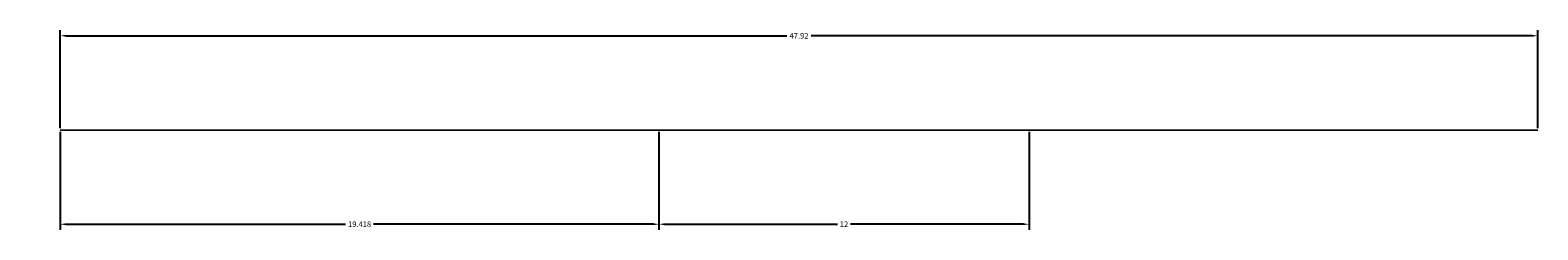
# Model space of a CAD drawing. Units: millimetres. Extents: x 4631 to 4863, y -3 to 1956.
# Tile 1 of 2: x 4814 to 4863, y -3 to 3. Entities that reach past the tile are written whole.
import ezdxf

# ---------------------------------------------------------------- set-up
doc = ezdxf.new("R2010")
doc.units = ezdxf.units.MM
doc.layers.add('M-CONS', color=8, linetype='Continuous', lineweight=13)
doc.layers.add('M-DIMS', color=2, linetype='Continuous', lineweight=18)
doc.styles.get("Standard").update_dxf_attribs({"font": 'arial.ttf'})
doc.dimstyles.get("Standard").update_dxf_attribs({"dimtxt": 0.18, "dimasz": 0.18, "dimexe": 0.18, "dimexo": 0.0625, "dimgap": 0.09, "dimtad": 0, "dimtih": 1, "dimtoh": 1, "dimdec": 4, "dimzin": 0, "dimdsep": 46, "dimtxsty": 'Standard', "dimcen": 0.09, "dimadec": 0, "dimazin": 0, "dimtfac": 1, "dimtdec": 4, "dimtofl": 0, "dimtmove": 0, "dimatfit": 3, "dimfxl": 1, "dimtolj": 1, "dimtzin": 0, "dimarcsym": 0})

# ---------------------------------------------------------------- blocks, each defined once
blk = doc.blocks.new('*D1')
at = {"layer": 'Defpoints', "color": 0, "transparency": 16777216}
for p in [(4863.262, 3.05), (4815.344, 0), (4863.262, 0)]:
    blk.add_point(p, dxfattribs=at)
at = {"layer": 'M-DIMS', "color": 0, "lineweight": -2, "transparency": 16777216}
for p, q in [((4815.344, 0.062), (4815.344, 3.23)), ((4815.524, 3.05), (4838.906, 3.05)), ((4863.082, 3.05), (4839.699, 3.05)), ((4863.262, 0.062), (4863.262, 3.23))]:
    blk.add_line(p, q, dxfattribs=at)
at = {"layer": 'M-DIMS', "color": 0, "transparency": 16777216}
for points in [[(4815.524, 3.08), (4815.524, 3.02), (4815.344, 3.05)], [(4863.082, 3.08), (4863.082, 3.02), (4863.262, 3.05)]]:
    blk.add_solid(points, dxfattribs=at)
at = {"layer": 'M-DIMS', "color": 0, "transparency": 16777216, "insert": (4839.303, 3.05), "char_height": 0.18, "attachment_point": 5}
blk.add_mtext('\\A1;47.92', dxfattribs=at)
blk = doc.blocks.new('*D2')
at = {"layer": 'Defpoints', "color": 0, "transparency": 16777216}
for p in [(4815.344, 0), (4834.762, 0), (4834.762, -3.05)]:
    blk.add_point(p, dxfattribs=at)
at = {"layer": 'M-DIMS', "color": 0, "lineweight": -2, "transparency": 16777216}
for p, q in [((4815.344, -0.062), (4815.344, -3.23)), ((4834.762, -0.062), (4834.762, -3.23)), ((4815.524, -3.05), (4824.597, -3.05)), ((4834.582, -3.05), (4825.508, -3.05))]:
    blk.add_line(p, q, dxfattribs=at)
at = {"layer": 'M-DIMS', "color": 0, "transparency": 16777216}
for points in [[(4815.524, -3.02), (4815.524, -3.08), (4815.344, -3.05)], [(4834.582, -3.02), (4834.582, -3.08), (4834.762, -3.05)]]:
    blk.add_solid(points, dxfattribs=at)
at = {"layer": 'M-DIMS', "color": 0, "transparency": 16777216, "insert": (4825.053, -3.05), "char_height": 0.18, "attachment_point": 5}
blk.add_mtext('\\A1;19.418', dxfattribs=at)
blk = doc.blocks.new('*D3')
at = {"layer": 'Defpoints', "color": 0, "transparency": 16777216}
for p in [(4834.762, 0), (4846.762, 0), (4846.762, -3.05)]:
    blk.add_point(p, dxfattribs=at)
at = {"layer": 'M-DIMS', "color": 0, "lineweight": -2, "transparency": 16777216}
for p, q in [((4834.762, -0.062), (4834.762, -3.23)), ((4846.762, -0.062), (4846.762, -3.23)), ((4834.942, -3.05), (4840.552, -3.05)), ((4846.582, -3.05), (4840.971, -3.05))]:
    blk.add_line(p, q, dxfattribs=at)
at = {"layer": 'M-DIMS', "color": 0, "transparency": 16777216}
for points in [[(4834.942, -3.02), (4834.942, -3.08), (4834.762, -3.05)], [(4846.582, -3.02), (4846.582, -3.08), (4846.762, -3.05)]]:
    blk.add_solid(points, dxfattribs=at)
at = {"layer": 'M-DIMS', "color": 0, "transparency": 16777216, "insert": (4840.762, -3.05), "char_height": 0.18, "attachment_point": 5}
blk.add_mtext('\\A1;12', dxfattribs=at)

msp = doc.modelspace()

# ---------------------------------------------------------------- linework, layer by layer
at = {"layer": 'M-CONS', "extrusion": (0, -1, 0)}
msp.add_lwpolyline([(4863.2618, -92.5722), (4818.2618, -92.5722, 0.145898), (4818.2618, -132.5722), (4863.2618, -132.5722)], format="xyb", close=True, dxfattribs=at)
msp.add_circle((4840.7618, -112.5722), 6, dxfattribs=at)

# ---------------------------------------------------------------- dimensions: what is measured, and where the dimension line sits
at = {"layer": 'M-DIMS'}
for base, p1, p2, override, picture, middle in [((4863.2618, 3.05), (4815.3438, 0), (4863.2618, 0), {"dimdec": 2, "dimlfac": 1, "dimrnd": 0, "dimzin": 0, "dimdsep": 46, "dimlunit": 2}, '*D1', (4839.3028, 3.05)), ((4834.7618, -3.05), (4815.3438, 0), (4834.7618, 0), {"dimdec": 3, "dimlfac": 1, "dimrnd": 0, "dimzin": 0, "dimdsep": 46, "dimlunit": 2}, '*D2', (4825.0528, -3.05)), ((4846.7618, -3.05), (4834.7618, 0), (4846.7618, 0), {"dimdec": 0, "dimlfac": 1, "dimrnd": 0, "dimzin": 0, "dimdsep": 46, "dimlunit": 2}, '*D3', (4840.7618, -3.05))]:
    dim = msp.add_linear_dim(base=base, p1=p1, p2=p2, dimstyle='Standard', override=override, dxfattribs=at)
    dim.commit()
    dim.dimension.update_dxf_attribs({"geometry": picture, "text_midpoint": middle})

doc.saveas('drawing.dxf')
